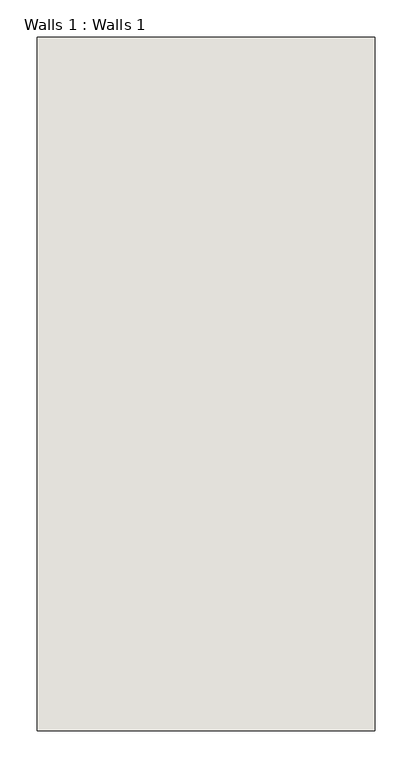
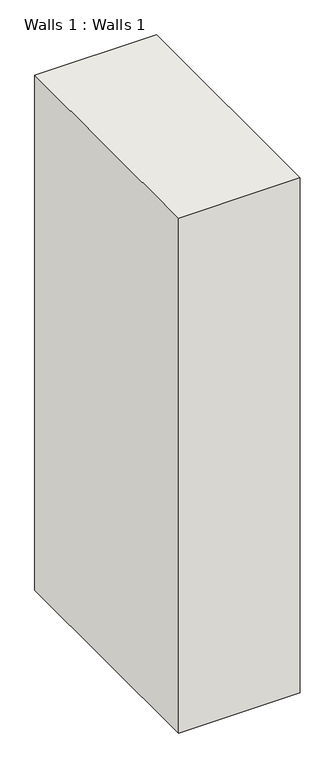
"""IFC4 building model written with IfcOpenShell, lengths in millimetres: wall geometry, Walls 1 : Walls 1."""

from ifc_helpers import new_model, si_unit, frame, origin, place, context, project, spatial, polyline, outline, extrude, faceted_brep, source, transform, mapped, element, save


def walls_1_walls_1_a7120c5c(model_context):
    return source(origin(), model_context, "Body", "SolidModel", [
        extrude(outline(polyline([(-8852.593556, -1272.981648), (-8852.593556, -2149.281648), (-9258.993556, -2149.281648), (-9258.993556, -1272.981648), (-8852.593556, -1272.981648)])), frame((0.0, 0.0, 574.7757913), z_axis=(0.0, 0.0, 1.0), x_axis=(1.0, 0.0, 0.0)), (0.0, 0.0, 1.0), 31.75),
        faceted_brep([(-8852.593556, -1237.4497499, 2198.6952722), (-8852.593556, -2174.681648, 2198.6952722), (-8852.593556, -2174.681648, 152.4), (-8852.593556, -1237.4497499, 152.4), (-8852.593556, -1262.8497499, 2173.2952722), (-8852.593556, -1262.8497499, 177.8), (-8852.593556, -2149.281648, 177.8), (-8852.593556, -2149.281648, 2173.2952722), (-9309.793556, -1237.4497499, 2198.6952722), (-9309.793556, -1237.4497499, 152.4), (-9309.793556, -2174.681648, 152.4), (-9309.793556, -2174.681648, 2198.6952722), (-9258.993556, -1262.8497499, 2173.2952722), (-9258.993556, -2149.281648, 2173.2952722), (-9258.993556, -2149.281648, 177.8), (-9258.993556, -1262.8497499, 177.8)], [[[0, 1, 2, 3], [4, 5, 6, 7]], [[8, 9, 10, 11]], [[1, 0, 8, 11]], [[2, 1, 11, 10]], [[3, 2, 10, 9]], [[0, 3, 9, 8]], [[12, 13, 14, 15]], [[12, 15, 5, 4]], [[15, 14, 6, 5]], [[14, 13, 7, 6]], [[13, 12, 4, 7]]]),
    ])


if __name__ == "__main__":
    model = new_model("IFC4")
    model_context = context("Model", 3, world=origin())
    ifc_project = project(units=[si_unit("LENGTHUNIT", "METRE", prefix="MILLI")], contexts=[model_context])
    site = spatial("IfcSite", under=ifc_project)
    building = spatial("IfcBuilding", under=site)
    placement = place(None, origin())
    walls_1_walls_1_shape = walls_1_walls_1_a7120c5c(model_context)
    element("IfcWall", 1, ObjectType="Walls 1 : Walls 1", at=placement, inside=building, context=model_context, shape_type="MappedRepresentation", body=[
        mapped(walls_1_walls_1_shape, transform((0.0, 0.0, 0.0), x_axis=(1.0, 0.0, 0.0), y_axis=(0.0, 1.0, 0.0), z_axis=(0.0, 0.0, 1.0))),
    ])
    save(model, "model.ifc")

# Revit data of these elements
# Element 1 (IfcWall, "Walls 1 : Walls 1")
#   Materials on its faces: "Default Wall"
# Materials
#   "Default Wall": colour RGB 128 128 128, transparency 0
